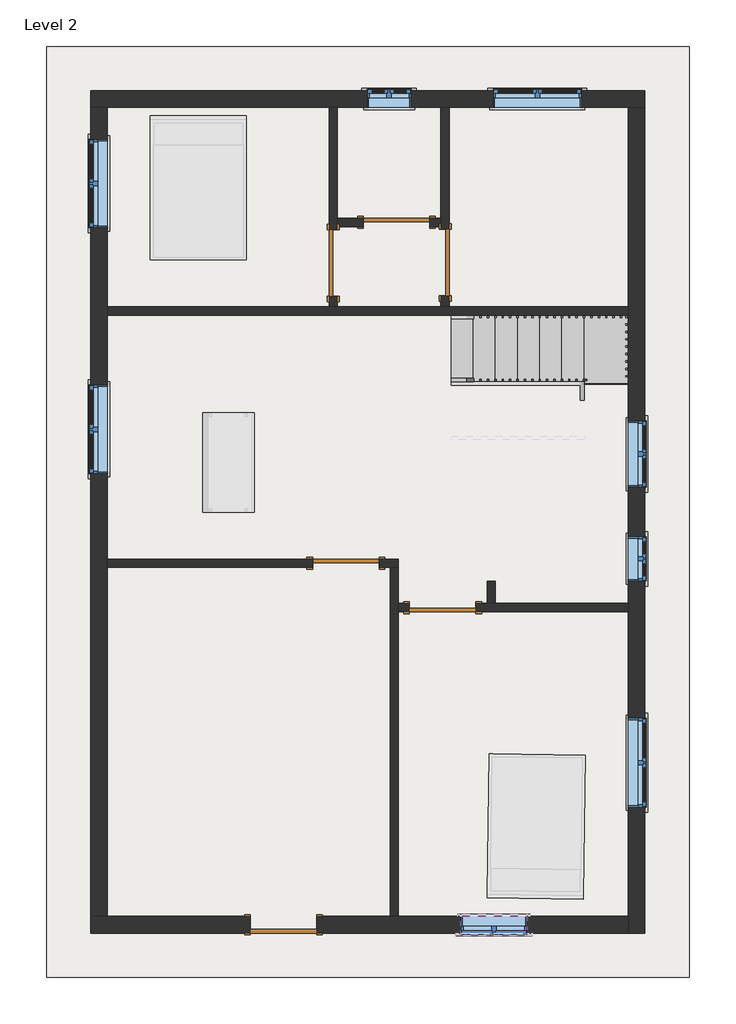
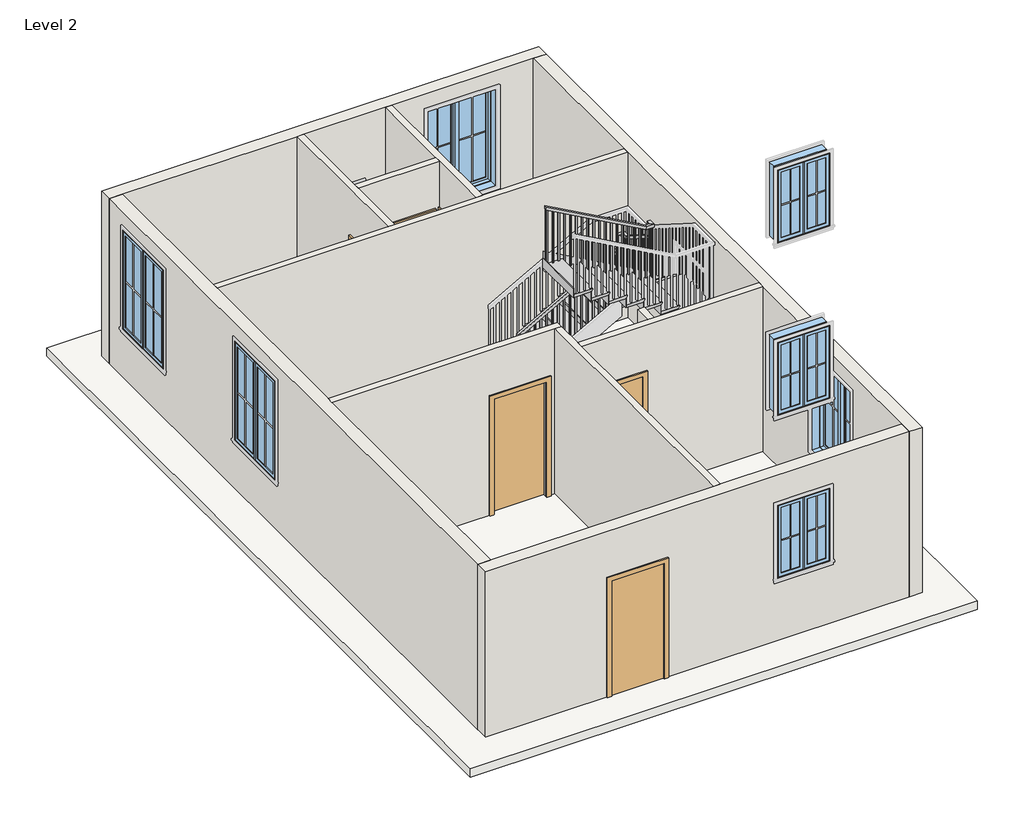
# One storey, part 1 of 2: 12 walls, 10 windows, 6 doors, 1 railing, 1 slab, 1 stair flight.
"""IFC4 building model written with IfcOpenShell, lengths in millimetres."""

from ifc_helpers import new_model, si_unit, frame, origin, place, context, project, spatial, polyline, outline, extrude, faceted_brep, transform, mapped, element, save
from components import door_e5f9f3c4, door_305aa2a5, door_0ca8825f, stair_flight_91d3489d, window_c417fced, window_79f73a1a, window_6ca1769e

model = new_model("IFC4")

# Units and contexts
model_context = context("Model", 3, world=origin())
ifc_project = project(units=[si_unit("LENGTHUNIT", "METRE", prefix="MILLI")], contexts=[model_context])

# Site, building, storey
site = spatial("IfcSite", under=ifc_project)
building = spatial("IfcBuilding", under=site)
storey = spatial("IfcBuildingStorey", under=building, Name="Level 2", Elevation=3048.0)

# Doors
placement = place(None, origin())
door_shape = door_e5f9f3c4(model_context)
element("IfcDoor", 1, ObjectType="Single-Flush : 36\" x 84\"", at=placement, inside=storey, context=model_context, shape_type="MappedRepresentation", body=[
    mapped(door_shape, transform((5727.7, 12245.5823212, 3048.0), x_axis=(1.0, 0.0, 0.0), y_axis=(0.0, 1.0, 0.0), z_axis=(0.0, 0.0, 1.0))),
])
element("IfcDoor", 2, ObjectType="Single-Flush : 36\" x 84\"", at=placement, inside=storey, context=model_context, shape_type="MappedRepresentation", body=[
    mapped(door_shape, transform((6394.45, 11693.1323212, 3048.0), x_axis=(0.0, -1.0, 0.0), y_axis=(1.0, 0.0, 0.0), z_axis=(0.0, 0.0, 1.0))),
])
element("IfcDoor", 3, ObjectType="Single-Flush : 36\" x 84\"", at=placement, inside=storey, context=model_context, shape_type="MappedRepresentation", body=[
    mapped(door_shape, transform((6362.7, 6949.6823212, 3048.0), x_axis=(-1.0, 0.0, 0.0), y_axis=(0.0, -1.0, 0.0), z_axis=(0.0, 0.0, 1.0))),
])
element("IfcDoor", 4, ObjectType="Single-Flush : 36\" x 84\"", at=placement, inside=storey, context=model_context, shape_type="MappedRepresentation", body=[
    mapped(door_shape, transform((5029.2, 7559.2823212, 3048.0), x_axis=(1.0, 0.0, 0.0), y_axis=(0.0, 1.0, 0.0), z_axis=(0.0, 0.0, 1.0))),
])
door_2_shape = door_305aa2a5(model_context)
element("IfcDoor", 5, ObjectType="Single-Flush : 36\" x 84\"", at=placement, inside=storey, context=model_context, shape_type="MappedRepresentation", body=[
    mapped(door_2_shape, transform((4857.75, 11689.9573212, 3048.0), x_axis=(0.0, -1.0, 0.0), y_axis=(1.0, 0.0, 0.0), z_axis=(0.0, 0.0, 1.0))),
])
door_3_shape = door_0ca8825f(model_context)
element("IfcDoor", 6, ObjectType="Single-Flush : 36\" x 84\"", at=placement, inside=storey, context=model_context, shape_type="MappedRepresentation", body=[
    mapped(door_3_shape, transform((4171.95, 2587.2323212, 3048.0), x_axis=(-1.0, 0.0, 0.0), y_axis=(0.0, -1.0, 0.0), z_axis=(0.0, 0.0, 1.0))),
])

# Railing
element("IfcRailing", 7, ObjectType="Handrail - Rectangular", at=placement, inside=storey, context=model_context, shape_type="SolidModel", body=[
    faceted_brep([(6477.0, 10105.6323212, 4131.7333333), (6477.0, 10105.6323212, 4073.620221), (6477.0, 10054.8323212, 4073.620221), (6477.0, 10054.8323212, 4131.7333333), (8229.6, 10105.6323212, 5105.4), (8280.4, 10105.6323212, 5075.5091099), (8280.4, 10054.8323212, 5075.5091099), (8229.6, 10054.8323212, 5105.4), (8229.6, 10105.6323212, 5365.447619), (8280.4, 10105.6323212, 5314.647619), (8280.4, 10054.8323212, 5314.647619), (8229.6, 10054.8323212, 5365.447619), (8356.6, 10105.6323212, 5365.447619), (8356.6, 10105.6323212, 5314.647619), (8305.8, 10054.8323212, 5314.647619), (8305.8, 10054.8323212, 5365.447619), (8356.6, 9978.6323212, 5365.447619), (8356.6, 9963.8676405, 5314.647619), (8305.8, 9963.8676405, 5314.647619), (8305.8, 9978.6323212, 5365.447619), (8356.6, 9330.9323212, 5776.6857143), (8356.6, 9280.1323212, 5748.7652821), (8305.8, 9280.1323212, 5748.7652821), (8305.8, 9330.9323212, 5776.6857143), (8356.6, 9330.9323212, 6036.7333333), (8356.6, 9280.1323212, 5985.9333333), (8305.8, 9280.1323212, 5985.9333333), (8305.8, 9330.9323212, 6036.7333333), (8356.6, 9203.9323212, 6036.7333333), (8356.6, 9203.9323212, 5985.9333333), (8305.8, 9254.7323212, 5985.9333333), (8305.8, 9254.7323212, 6036.7333333), (8229.6, 9203.9323212, 6036.7333333), (8216.4363978, 9203.9323212, 5985.9333333), (8216.4363978, 9254.7323212, 5985.9333333), (8229.6, 9254.7323212, 6036.7333333), (6477.0, 9203.9323212, 7010.4), (6477.0, 9254.7323212, 7010.4), (6477.0, 9254.7323212, 6952.2868876), (6477.0, 9203.9323212, 6952.2868876)], [[[0, 1, 2, 3]], [[1, 0, 4, 5]], [[2, 1, 5, 6]], [[3, 2, 6, 7]], [[0, 3, 7, 4]], [[5, 4, 8, 9]], [[6, 5, 9, 10]], [[7, 6, 10, 11]], [[4, 7, 11, 8]], [[9, 8, 12, 13]], [[10, 9, 13, 14]], [[11, 10, 14, 15]], [[8, 11, 15, 12]], [[13, 12, 16, 17]], [[14, 13, 17, 18]], [[15, 14, 18, 19]], [[12, 15, 19, 16]], [[17, 16, 20, 21]], [[18, 17, 21, 22]], [[19, 18, 22, 23]], [[16, 19, 23, 20]], [[21, 20, 24, 25]], [[22, 21, 25, 26]], [[23, 22, 26, 27]], [[20, 23, 27, 24]], [[25, 24, 28, 29]], [[26, 25, 29, 30]], [[27, 26, 30, 31]], [[24, 27, 31, 28]], [[29, 28, 32, 33]], [[30, 29, 33, 34]], [[31, 30, 34, 35]], [[28, 31, 35, 32]], [[36, 37, 38, 39]], [[33, 32, 36, 39]], [[34, 33, 39, 38]], [[35, 34, 38, 37]], [[32, 35, 37, 36]]]),
    extrude(outline(polyline([(6932.8841099, 6511.925), (6943.4674432, 6492.875), (5926.6666667, 6492.875), (5926.6666667, 6511.925), (6932.8841099, 6511.925)])), frame((0.0, 9219.8073212, 0.0), z_axis=(0.0, 1.0, 0.0), x_axis=(0.0, 0.0, 1.0)), (0.0, 0.0, 1.0), 19.05),
    extrude(outline(polyline([(6876.4396654, 6613.525), (6887.0229988, 6594.475), (5926.6666667, 6594.475), (5926.6666667, 6613.525), (6876.4396654, 6613.525)])), frame((0.0, 9219.8073212, 0.0), z_axis=(0.0, 1.0, 0.0), x_axis=(0.0, 0.0, 1.0)), (0.0, 0.0, 1.0), 19.05),
    extrude(outline(polyline([(6819.995221, 6715.125), (6830.5785543, 6696.075), (5926.6666667, 6696.075), (5926.6666667, 6715.125), (6819.995221, 6715.125)])), frame((0.0, 9219.8073212, 0.0), z_axis=(0.0, 1.0, 0.0), x_axis=(0.0, 0.0, 1.0)), (0.0, 0.0, 1.0), 19.05),
    extrude(outline(polyline([(6763.5507765, 6816.725), (6774.1341099, 6797.675), (5757.3333333, 6797.675), (5757.3333333, 6816.725), (6763.5507765, 6816.725)])), frame((0.0, 9219.8073212, 0.0), z_axis=(0.0, 1.0, 0.0), x_axis=(0.0, 0.0, 1.0)), (0.0, 0.0, 1.0), 19.05),
    extrude(outline(polyline([(6707.1063321, 6918.325), (6717.6896654, 6899.275), (5757.3333333, 6899.275), (5757.3333333, 6918.325), (6707.1063321, 6918.325)])), frame((0.0, 9219.8073212, 0.0), z_axis=(0.0, 1.0, 0.0), x_axis=(0.0, 0.0, 1.0)), (0.0, 0.0, 1.0), 19.05),
    extrude(outline(polyline([(6650.6618876, 7019.925), (6661.245221, 7000.875), (5757.3333333, 7000.875), (5757.3333333, 7019.925), (6650.6618876, 7019.925)])), frame((0.0, 9219.8073212, 0.0), z_axis=(0.0, 1.0, 0.0), x_axis=(0.0, 0.0, 1.0)), (0.0, 0.0, 1.0), 19.05),
    extrude(outline(polyline([(6594.2174432, 7121.525), (6604.8007765, 7102.475), (5588.0, 7102.475), (5588.0, 7121.525), (6594.2174432, 7121.525)])), frame((0.0, 9219.8073212, 0.0), z_axis=(0.0, 1.0, 0.0), x_axis=(0.0, 0.0, 1.0)), (0.0, 0.0, 1.0), 19.05),
    extrude(outline(polyline([(6537.7729988, 7223.125), (6548.3563321, 7204.075), (5588.0, 7204.075), (5588.0, 7223.125), (6537.7729988, 7223.125)])), frame((0.0, 9219.8073212, 0.0), z_axis=(0.0, 1.0, 0.0), x_axis=(0.0, 0.0, 1.0)), (0.0, 0.0, 1.0), 19.05),
    extrude(outline(polyline([(6481.3285543, 7324.725), (6491.9118876, 7305.675), (5588.0, 7305.675), (5588.0, 7324.725), (6481.3285543, 7324.725)])), frame((0.0, 9219.8073212, 0.0), z_axis=(0.0, 1.0, 0.0), x_axis=(0.0, 0.0, 1.0)), (0.0, 0.0, 1.0), 19.05),
    extrude(outline(polyline([(6424.8841099, 7426.325), (6435.4674432, 7407.275), (5418.6666667, 7407.275), (5418.6666667, 7426.325), (6424.8841099, 7426.325)])), frame((0.0, 9219.8073212, 0.0), z_axis=(0.0, 1.0, 0.0), x_axis=(0.0, 0.0, 1.0)), (0.0, 0.0, 1.0), 19.05),
    extrude(outline(polyline([(6368.4396654, 7527.925), (6379.0229988, 7508.875), (5418.6666667, 7508.875), (5418.6666667, 7527.925), (6368.4396654, 7527.925)])), frame((0.0, 9219.8073212, 0.0), z_axis=(0.0, 1.0, 0.0), x_axis=(0.0, 0.0, 1.0)), (0.0, 0.0, 1.0), 19.05),
    extrude(outline(polyline([(6311.995221, 7629.525), (6322.5785543, 7610.475), (5418.6666667, 7610.475), (5418.6666667, 7629.525), (6311.995221, 7629.525)])), frame((0.0, 9219.8073212, 0.0), z_axis=(0.0, 1.0, 0.0), x_axis=(0.0, 0.0, 1.0)), (0.0, 0.0, 1.0), 19.05),
    extrude(outline(polyline([(6255.5507765, 7731.125), (6266.1341099, 7712.075), (5249.3333333, 7712.075), (5249.3333333, 7731.125), (6255.5507765, 7731.125)])), frame((0.0, 9219.8073212, 0.0), z_axis=(0.0, 1.0, 0.0), x_axis=(0.0, 0.0, 1.0)), (0.0, 0.0, 1.0), 19.05),
    extrude(outline(polyline([(6199.1063321, 7832.725), (6209.6896654, 7813.675), (5249.3333333, 7813.675), (5249.3333333, 7832.725), (6199.1063321, 7832.725)])), frame((0.0, 9219.8073212, 0.0), z_axis=(0.0, 1.0, 0.0), x_axis=(0.0, 0.0, 1.0)), (0.0, 0.0, 1.0), 19.05),
    extrude(outline(polyline([(6142.6618876, 7934.325), (6153.245221, 7915.275), (5249.3333333, 7915.275), (5249.3333333, 7934.325), (6142.6618876, 7934.325)])), frame((0.0, 9219.8073212, 0.0), z_axis=(0.0, 1.0, 0.0), x_axis=(0.0, 0.0, 1.0)), (0.0, 0.0, 1.0), 19.05),
    extrude(outline(polyline([(6086.2174432, 8035.925), (6096.8007765, 8016.875), (5080.0, 8016.875), (5080.0, 8035.925), (6086.2174432, 8035.925)])), frame((0.0, 9219.8073212, 0.0), z_axis=(0.0, 1.0, 0.0), x_axis=(0.0, 0.0, 1.0)), (0.0, 0.0, 1.0), 19.05),
    extrude(outline(polyline([(6029.7729988, 8137.525), (6040.3563321, 8118.475), (5080.0, 8118.475), (5080.0, 8137.525), (6029.7729988, 8137.525)])), frame((0.0, 9219.8073212, 0.0), z_axis=(0.0, 1.0, 0.0), x_axis=(0.0, 0.0, 1.0)), (0.0, 0.0, 1.0), 19.05),
    extrude(outline(polyline([(5973.3285543, 8239.125), (5983.9118876, 8220.075), (5080.0, 8220.075), (5080.0, 8239.125), (5973.3285543, 8239.125)])), frame((0.0, 9219.8073212, 0.0), z_axis=(0.0, 1.0, 0.0), x_axis=(0.0, 0.0, 1.0)), (0.0, 0.0, 1.0), 19.05),
    extrude(outline(polyline([(8321.675, 9276.9573212), (8340.725, 9276.9573212), (8340.725, 9257.9073212), (8321.675, 9257.9073212), (8321.675, 9276.9573212)])), frame((0.0, 0.0, 4741.3333333), z_axis=(0.0, 0.0, 1.0), x_axis=(1.0, 0.0, 0.0)), (0.0, 0.0, 1.0), 1244.6),
    extrude(outline(polyline([(9359.5073212, 5698.3684567), (9378.5573212, 5686.2732186), (9378.5573212, 4741.3333333), (9359.5073212, 4741.3333333), (9359.5073212, 5698.3684567)])), frame((8321.675, 0.0, 0.0), z_axis=(1.0, 0.0, 0.0), x_axis=(0.0, 1.0, 0.0)), (0.0, 0.0, 1.0), 19.05),
    extrude(outline(polyline([(9461.1073212, 5633.8605202), (9480.1573212, 5621.7652821), (9480.1573212, 4741.3333333), (9461.1073212, 4741.3333333), (9461.1073212, 5633.8605202)])), frame((8321.675, 0.0, 0.0), z_axis=(1.0, 0.0, 0.0), x_axis=(0.0, 1.0, 0.0)), (0.0, 0.0, 1.0), 19.05),
    extrude(outline(polyline([(9562.7073212, 5569.3525837), (9581.7573212, 5557.2573456), (9581.7573212, 4572.0), (9562.7073212, 4572.0), (9562.7073212, 5569.3525837)])), frame((8321.675, 0.0, 0.0), z_axis=(1.0, 0.0, 0.0), x_axis=(0.0, 1.0, 0.0)), (0.0, 0.0, 1.0), 19.05),
    extrude(outline(polyline([(9664.3073212, 5504.8446472), (9683.3573212, 5492.7494091), (9683.3573212, 4572.0), (9664.3073212, 4572.0), (9664.3073212, 5504.8446472)])), frame((8321.675, 0.0, 0.0), z_axis=(1.0, 0.0, 0.0), x_axis=(0.0, 1.0, 0.0)), (0.0, 0.0, 1.0), 19.05),
    extrude(outline(polyline([(9765.9073212, 5440.3367107), (9784.9573212, 5428.2414726), (9784.9573212, 4402.6666667), (9765.9073212, 4402.6666667), (9765.9073212, 5440.3367107)])), frame((8321.675, 0.0, 0.0), z_axis=(1.0, 0.0, 0.0), x_axis=(0.0, 1.0, 0.0)), (0.0, 0.0, 1.0), 19.05),
    extrude(outline(polyline([(9867.5073212, 5375.8287742), (9886.5573212, 5363.7335361), (9886.5573212, 4402.6666667), (9867.5073212, 4402.6666667), (9867.5073212, 5375.8287742)])), frame((8321.675, 0.0, 0.0), z_axis=(1.0, 0.0, 0.0), x_axis=(0.0, 1.0, 0.0)), (0.0, 0.0, 1.0), 19.05),
    extrude(outline(polyline([(9969.1073212, 5311.3208377), (9988.1573212, 5299.2255996), (9988.1573212, 4402.6666667), (9969.1073212, 4402.6666667), (9969.1073212, 5311.3208377)])), frame((8321.675, 0.0, 0.0), z_axis=(1.0, 0.0, 0.0), x_axis=(0.0, 1.0, 0.0)), (0.0, 0.0, 1.0), 19.05),
    extrude(outline(polyline([(8296.275, 10070.7073212), (8296.275, 10089.7573212), (8315.325, 10089.7573212), (8315.325, 10070.7073212), (8296.275, 10070.7073212)])), frame((0.0, 0.0, 4233.3333333), z_axis=(0.0, 0.0, 1.0), x_axis=(1.0, 0.0, 0.0)), (0.0, 0.0, 1.0), 1081.3142857),
    extrude(outline(polyline([(5038.4674432, 8213.725), (5027.8841099, 8194.675), (4064.0, 8194.675), (4064.0, 8213.725), (5038.4674432, 8213.725)])), frame((0.0, 10070.7073212, 0.0), z_axis=(0.0, 1.0, 0.0), x_axis=(0.0, 0.0, 1.0)), (0.0, 0.0, 1.0), 19.05),
    extrude(outline(polyline([(4982.0229988, 8112.125), (4971.4396654, 8093.075), (4064.0, 8093.075), (4064.0, 8112.125), (4982.0229988, 8112.125)])), frame((0.0, 10070.7073212, 0.0), z_axis=(0.0, 1.0, 0.0), x_axis=(0.0, 0.0, 1.0)), (0.0, 0.0, 1.0), 19.05),
    extrude(outline(polyline([(4925.5785543, 8010.525), (4914.995221, 7991.475), (4064.0, 7991.475), (4064.0, 8010.525), (4925.5785543, 8010.525)])), frame((0.0, 10070.7073212, 0.0), z_axis=(0.0, 1.0, 0.0), x_axis=(0.0, 0.0, 1.0)), (0.0, 0.0, 1.0), 19.05),
    extrude(outline(polyline([(4869.1341099, 7908.925), (4858.5507765, 7889.875), (3894.6666667, 7889.875), (3894.6666667, 7908.925), (4869.1341099, 7908.925)])), frame((0.0, 10070.7073212, 0.0), z_axis=(0.0, 1.0, 0.0), x_axis=(0.0, 0.0, 1.0)), (0.0, 0.0, 1.0), 19.05),
    extrude(outline(polyline([(4812.6896654, 7807.325), (4802.1063321, 7788.275), (3894.6666667, 7788.275), (3894.6666667, 7807.325), (4812.6896654, 7807.325)])), frame((0.0, 10070.7073212, 0.0), z_axis=(0.0, 1.0, 0.0), x_axis=(0.0, 0.0, 1.0)), (0.0, 0.0, 1.0), 19.05),
    extrude(outline(polyline([(4756.245221, 7705.725), (4745.6618876, 7686.675), (3894.6666667, 7686.675), (3894.6666667, 7705.725), (4756.245221, 7705.725)])), frame((0.0, 10070.7073212, 0.0), z_axis=(0.0, 1.0, 0.0), x_axis=(0.0, 0.0, 1.0)), (0.0, 0.0, 1.0), 19.05),
    extrude(outline(polyline([(4699.8007765, 7604.125), (4689.2174432, 7585.075), (3725.3333333, 7585.075), (3725.3333333, 7604.125), (4699.8007765, 7604.125)])), frame((0.0, 10070.7073212, 0.0), z_axis=(0.0, 1.0, 0.0), x_axis=(0.0, 0.0, 1.0)), (0.0, 0.0, 1.0), 19.05),
    extrude(outline(polyline([(4643.3563321, 7502.525), (4632.7729988, 7483.475), (3725.3333333, 7483.475), (3725.3333333, 7502.525), (4643.3563321, 7502.525)])), frame((0.0, 10070.7073212, 0.0), z_axis=(0.0, 1.0, 0.0), x_axis=(0.0, 0.0, 1.0)), (0.0, 0.0, 1.0), 19.05),
    extrude(outline(polyline([(4586.9118876, 7400.925), (4576.3285543, 7381.875), (3725.3333333, 7381.875), (3725.3333333, 7400.925), (4586.9118876, 7400.925)])), frame((0.0, 10070.7073212, 0.0), z_axis=(0.0, 1.0, 0.0), x_axis=(0.0, 0.0, 1.0)), (0.0, 0.0, 1.0), 19.05),
    extrude(outline(polyline([(4530.4674432, 7299.325), (4519.8841099, 7280.275), (3556.0, 7280.275), (3556.0, 7299.325), (4530.4674432, 7299.325)])), frame((0.0, 10070.7073212, 0.0), z_axis=(0.0, 1.0, 0.0), x_axis=(0.0, 0.0, 1.0)), (0.0, 0.0, 1.0), 19.05),
    extrude(outline(polyline([(4474.0229988, 7197.725), (4463.4396654, 7178.675), (3556.0, 7178.675), (3556.0, 7197.725), (4474.0229988, 7197.725)])), frame((0.0, 10070.7073212, 0.0), z_axis=(0.0, 1.0, 0.0), x_axis=(0.0, 0.0, 1.0)), (0.0, 0.0, 1.0), 19.05),
    extrude(outline(polyline([(4417.5785543, 7096.125), (4406.995221, 7077.075), (3556.0, 7077.075), (3556.0, 7096.125), (4417.5785543, 7096.125)])), frame((0.0, 10070.7073212, 0.0), z_axis=(0.0, 1.0, 0.0), x_axis=(0.0, 0.0, 1.0)), (0.0, 0.0, 1.0), 19.05),
    extrude(outline(polyline([(4361.1341099, 6994.525), (4350.5507765, 6975.475), (3386.6666667, 6975.475), (3386.6666667, 6994.525), (4361.1341099, 6994.525)])), frame((0.0, 10070.7073212, 0.0), z_axis=(0.0, 1.0, 0.0), x_axis=(0.0, 0.0, 1.0)), (0.0, 0.0, 1.0), 19.05),
    extrude(outline(polyline([(4304.6896654, 6892.925), (4294.1063321, 6873.875), (3386.6666667, 6873.875), (3386.6666667, 6892.925), (4304.6896654, 6892.925)])), frame((0.0, 10070.7073212, 0.0), z_axis=(0.0, 1.0, 0.0), x_axis=(0.0, 0.0, 1.0)), (0.0, 0.0, 1.0), 19.05),
    extrude(outline(polyline([(4248.245221, 6791.325), (4237.6618876, 6772.275), (3386.6666667, 6772.275), (3386.6666667, 6791.325), (4248.245221, 6791.325)])), frame((0.0, 10070.7073212, 0.0), z_axis=(0.0, 1.0, 0.0), x_axis=(0.0, 0.0, 1.0)), (0.0, 0.0, 1.0), 19.05),
    extrude(outline(polyline([(4191.8007765, 6689.725), (4181.2174432, 6670.675), (3217.3333333, 6670.675), (3217.3333333, 6689.725), (4191.8007765, 6689.725)])), frame((0.0, 10070.7073212, 0.0), z_axis=(0.0, 1.0, 0.0), x_axis=(0.0, 0.0, 1.0)), (0.0, 0.0, 1.0), 19.05),
    extrude(outline(polyline([(4135.3563321, 6588.125), (4124.7729988, 6569.075), (3217.3333333, 6569.075), (3217.3333333, 6588.125), (4135.3563321, 6588.125)])), frame((0.0, 10070.7073212, 0.0), z_axis=(0.0, 1.0, 0.0), x_axis=(0.0, 0.0, 1.0)), (0.0, 0.0, 1.0), 19.05),
    extrude(outline(polyline([(8321.675, 9238.8573212), (8340.725, 9238.8573212), (8340.725, 9219.8073212), (8321.675, 9219.8073212), (8321.675, 9238.8573212)])), frame((0.0, 0.0, 4910.6666667), z_axis=(0.0, 0.0, 1.0), x_axis=(1.0, 0.0, 0.0)), (0.0, 0.0, 1.0), 1075.2666667),
    extrude(outline(polyline([(8321.675, 10070.7073212), (8321.675, 10089.7573212), (8340.725, 10089.7573212), (8340.725, 10070.7073212), (8321.675, 10070.7073212)])), frame((0.0, 0.0, 4233.3333333), z_axis=(0.0, 0.0, 1.0), x_axis=(1.0, 0.0, 0.0)), (0.0, 0.0, 1.0), 1081.3142857),
    extrude(outline(polyline([(6941.7035543, 6496.05), (6952.2868876, 6477.0), (5926.6666667, 6477.0), (5926.6666667, 6496.05), (6941.7035543, 6496.05)])), frame((0.0, 9219.8073212, 0.0), z_axis=(0.0, 1.0, 0.0), x_axis=(0.0, 0.0, 1.0)), (0.0, 0.0, 1.0), 19.05),
    extrude(outline(polyline([(4084.2035543, 6496.05), (4073.620221, 6477.0), (3217.3333333, 6477.0), (3217.3333333, 6496.05), (4084.2035543, 6496.05)])), frame((0.0, 10070.7073212, 0.0), z_axis=(0.0, 1.0, 0.0), x_axis=(0.0, 0.0, 1.0)), (0.0, 0.0, 1.0), 19.05),
])

# Slab
element("IfcSlab", 8, ObjectType="Generic - 12\"", at=placement, inside=storey, context=model_context, shape_type="SweptSolid", body=[
    extrude(outline(polyline([(9753.6, 14664.9323212), (9753.6, 1863.3323212), (914.4, 1863.3323212), (914.4, 14664.9323212), (9753.6, 14664.9323212)])), frame((0.0, 0.0, 2895.6), z_axis=(0.0, 0.0, 1.0), x_axis=(1.0, 0.0, 0.0)), (0.0, 0.0, 1.0), 152.4),
])

# Stair flight
stair_flight_shape = stair_flight_91d3489d(model_context)
element("IfcStairFlight", 9, ObjectType="2\" Tread 1\" Nosing 1/4\" Riser", at=placement, inside=storey, context=model_context, shape_type="MappedRepresentation", body=[
    mapped(stair_flight_shape, transform((0.0, 0.0, 0.0), x_axis=(1.0, 0.0, 0.0), y_axis=(0.0, 1.0, 0.0), z_axis=(0.0, 0.0, 1.0))),
])

# Walls
element("IfcWall", 10, ObjectType="Generic - 5\"", at=placement, inside=storey, context=model_context, shape_type="Brep", body=[
    faceted_brep([(4800.6, 11232.7573212, 5181.6), (4800.6, 11232.7573212, 3048.0), (4800.6, 11083.5323212, 3048.0), (4800.6, 11083.5323212, 6096.0), (4800.6, 13826.7323212, 6096.0), (4800.6, 13826.7323212, 3048.0), (4800.6, 12147.1573212, 3048.0), (4800.6, 12147.1573212, 5181.6), (4914.9, 11083.5323212, 3048.0), (4914.9, 11232.7573212, 3048.0), (4914.9, 11232.7573212, 5181.6), (4914.9, 12147.1573212, 5181.6), (4914.9, 12147.1573212, 3048.0), (4914.9, 12188.4323212, 3048.0), (4914.9, 12302.7323212, 3048.0), (4914.9, 13826.7323212, 3048.0), (4914.9, 13826.7323212, 6096.0), (4914.9, 12302.7323212, 6096.0), (4914.9, 12188.4323212, 6096.0), (4914.9, 11083.5323212, 6096.0)], [[[0, 1, 2, 3, 4, 5, 6, 7]], [[8, 9, 10, 11, 12, 13, 14, 15, 16, 17, 18, 19]], [[6, 5, 15, 14, 13, 12]], [[2, 1, 9, 8]], [[4, 3, 19, 18, 17, 16]], [[5, 4, 16, 15]], [[3, 2, 8, 19]], [[10, 9, 1, 0]], [[11, 10, 0, 7]], [[12, 11, 7, 6]]]),
])
element("IfcWall", 11, ObjectType="Generic - 5\"", at=placement, inside=storey, context=model_context, shape_type="Brep", body=[
    faceted_brep([(6337.3, 11235.9323212, 5181.6), (6337.3, 11235.9323212, 3048.0), (6337.3, 11083.5323212, 3048.0), (6337.3, 11083.5323212, 6096.0), (6337.3, 12188.4323212, 6096.0), (6337.3, 12302.7323212, 6096.0), (6337.3, 13826.7323212, 6096.0), (6337.3, 13826.7323212, 3048.0), (6337.3, 12302.7323212, 3048.0), (6337.3, 12188.4323212, 3048.0), (6337.3, 12150.3323212, 3048.0), (6337.3, 12150.3323212, 5181.6), (6451.6, 11083.5323212, 3048.0), (6451.6, 11235.9323212, 3048.0), (6451.6, 11235.9323212, 5181.6), (6451.6, 12150.3323212, 5181.6), (6451.6, 12150.3323212, 3048.0), (6451.6, 13826.7323212, 3048.0), (6451.6, 13826.7323212, 6096.0), (6451.6, 11083.5323212, 6096.0)], [[[0, 1, 2, 3, 4, 5, 6, 7, 8, 9, 10, 11]], [[12, 13, 14, 15, 16, 17, 18, 19]], [[2, 1, 13, 12]], [[10, 9, 8, 7, 17, 16]], [[6, 5, 4, 3, 19, 18]], [[7, 6, 18, 17]], [[3, 2, 12, 19]], [[14, 13, 1, 0]], [[15, 14, 0, 11]], [[16, 15, 11, 10]]]),
])
element("IfcWall", 12, ObjectType="Generic - 5\"", at=placement, inside=storey, context=model_context, shape_type="SweptSolid", body=[
    extrude(outline(polyline([(5181.6, 6184.9), (3048.0, 6184.9), (3048.0, 6337.3), (6096.0, 6337.3), (6096.0, 4914.9), (3048.0, 4914.9), (3048.0, 5270.5), (5181.6, 5270.5), (5181.6, 6184.9)])), frame((0.0, 12188.4323212, 0.0), z_axis=(0.0, 1.0, 0.0), x_axis=(0.0, 0.0, 1.0)), (0.0, 0.0, 1.0), 114.3),
])
element("IfcWall", 13, ObjectType="Generic - 5\"", at=placement, inside=storey, context=model_context, shape_type="Brep", body=[
    faceted_brep([(1752.6, 10969.2323212, 3048.0), (8915.4, 10969.2323212, 3048.0), (8915.4, 10969.2323212, 6096.0), (1752.6, 10969.2323212, 6096.0), (1752.6, 11083.5323212, 3048.0), (1752.6, 11083.5323212, 6096.0), (4800.6, 11083.5323212, 6096.0), (4914.9, 11083.5323212, 6096.0), (6337.3, 11083.5323212, 6096.0), (6451.6, 11083.5323212, 6096.0), (8915.4, 11083.5323212, 6096.0), (8915.4, 11083.5323212, 3048.0), (6451.6, 11083.5323212, 3048.0), (6337.3, 11083.5323212, 3048.0), (4914.9, 11083.5323212, 3048.0), (4800.6, 11083.5323212, 3048.0)], [[[0, 1, 2, 3]], [[4, 5, 6, 7, 8, 9, 10, 11, 12, 13, 14, 15]], [[1, 0, 4, 15, 14, 13, 12, 11]], [[3, 2, 10, 9, 8, 7, 6, 5]], [[2, 1, 11, 10]], [[0, 3, 5, 4]]]),
])
element("IfcWall", 14, ObjectType="Generic - 5\"", at=placement, inside=storey, context=model_context, shape_type="Brep", body=[
    faceted_brep([(5486.4, 7502.1323212, 5181.6), (5486.4, 7502.1323212, 3048.0), (5638.8, 7502.1323212, 3048.0), (5753.1, 7502.1323212, 3048.0), (5753.1, 7502.1323212, 6096.0), (5638.8, 7502.1323212, 6096.0), (1752.6, 7502.1323212, 6096.0), (1752.6, 7502.1323212, 3048.0), (4572.0, 7502.1323212, 3048.0), (4572.0, 7502.1323212, 5181.6), (5753.1, 7616.4323212, 3048.0), (5486.4, 7616.4323212, 3048.0), (5486.4, 7616.4323212, 5181.6), (4572.0, 7616.4323212, 5181.6), (4572.0, 7616.4323212, 3048.0), (1752.6, 7616.4323212, 3048.0), (1752.6, 7616.4323212, 6096.0), (5753.1, 7616.4323212, 6096.0)], [[[0, 1, 2, 3, 4, 5, 6, 7, 8, 9]], [[10, 11, 12, 13, 14, 15, 16, 17]], [[8, 7, 15, 14]], [[3, 2, 1, 11, 10]], [[6, 5, 4, 17, 16]], [[7, 6, 16, 15]], [[4, 3, 10, 17]], [[12, 11, 1, 0]], [[13, 12, 0, 9]], [[14, 13, 9, 8]]]),
])
element("IfcWall", 15, ObjectType="Generic - 5\"", at=placement, inside=storey, context=model_context, shape_type="Brep", body=[
    faceted_brep([(5638.8, 7502.1323212, 3048.0), (5638.8, 2701.5323212, 3048.0), (5638.8, 2701.5323212, 6096.0), (5638.8, 7502.1323212, 6096.0), (5753.1, 7502.1323212, 3048.0), (5753.1, 7502.1323212, 6096.0), (5753.1, 7006.8323212, 6096.0), (5753.1, 6892.5323212, 6096.0), (5753.1, 2701.5323212, 6096.0), (5753.1, 2701.5323212, 3048.0), (5753.1, 6892.5323212, 3048.0), (5753.1, 7006.8323212, 3048.0)], [[[0, 1, 2, 3]], [[4, 5, 6, 7, 8, 9, 10, 11]], [[1, 0, 4, 11, 10, 9]], [[3, 2, 8, 7, 6, 5]], [[0, 3, 5, 4]], [[2, 1, 9, 8]]]),
])
element("IfcWall", 16, ObjectType="Generic - 5\"", at=placement, inside=storey, context=model_context, shape_type="Brep", body=[
    faceted_brep([(5905.5, 7006.8323212, 5181.6), (5905.5, 7006.8323212, 3048.0), (5753.1, 7006.8323212, 3048.0), (5753.1, 7006.8323212, 6096.0), (6972.3, 7006.8323212, 6096.0), (7086.6, 7006.8323212, 6096.0), (8915.4, 7006.8323212, 6096.0), (8915.4, 7006.8323212, 3048.0), (7086.6, 7006.8323212, 3048.0), (6972.3, 7006.8323212, 3048.0), (6819.9, 7006.8323212, 3048.0), (6819.9, 7006.8323212, 5181.6), (5753.1, 6892.5323212, 3048.0), (5905.5, 6892.5323212, 3048.0), (5905.5, 6892.5323212, 5181.6), (6819.9, 6892.5323212, 5181.6), (6819.9, 6892.5323212, 3048.0), (8915.4, 6892.5323212, 3048.0), (8915.4, 6892.5323212, 6096.0), (5753.1, 6892.5323212, 6096.0)], [[[0, 1, 2, 3, 4, 5, 6, 7, 8, 9, 10, 11]], [[12, 13, 14, 15, 16, 17, 18, 19]], [[2, 1, 13, 12]], [[10, 9, 8, 7, 17, 16]], [[6, 5, 4, 3, 19, 18]], [[7, 6, 18, 17]], [[3, 2, 12, 19]], [[14, 13, 1, 0]], [[15, 14, 0, 11]], [[16, 15, 11, 10]]]),
])
element("IfcWall", 17, ObjectType="Generic - 5\"", at=placement, inside=storey, context=model_context, shape_type="SweptSolid", body=[
    extrude(outline(polyline([(7086.6, 7311.6323212), (7086.6, 7006.8323212), (6972.3, 7006.8323212), (6972.3, 7311.6323212), (7086.6, 7311.6323212)])), frame((0.0, 0.0, 3048.0), z_axis=(0.0, 0.0, 1.0), x_axis=(1.0, 0.0, 0.0)), (0.0, 0.0, 1.0), 3048.0),
])
element("IfcWall", 18, ObjectType="Generic - 8\"", at=placement, inside=storey, context=model_context, shape_type="Brep", body=[
    faceted_brep([(1524.0, 13826.7323212, 3048.0), (1752.6, 13826.7323212, 3048.0), (4800.6, 13826.7323212, 3048.0), (4914.9, 13826.7323212, 3048.0), (6337.3, 13826.7323212, 3048.0), (6451.6, 13826.7323212, 3048.0), (8915.4, 13826.7323212, 3048.0), (9144.0, 13826.7323212, 3048.0), (9144.0, 13826.7323212, 6096.0), (8915.4, 13826.7323212, 6096.0), (6451.6, 13826.7323212, 6096.0), (6337.3, 13826.7323212, 6096.0), (4914.9, 13826.7323212, 6096.0), (4800.6, 13826.7323212, 6096.0), (1752.6, 13826.7323212, 6096.0), (1524.0, 13826.7323212, 6096.0), (8274.05, 13826.7323212, 5791.2), (8274.05, 13826.7323212, 3962.4), (7054.85, 13826.7323212, 3962.4), (7054.85, 13826.7323212, 5791.2), (5930.9, 13826.7323212, 4876.8), (5930.9, 13826.7323212, 3962.4), (5321.3, 13826.7323212, 3962.4), (5321.3, 13826.7323212, 4876.8), (1524.0, 14055.3323212, 3048.0), (1524.0, 14055.3323212, 6096.0), (9144.0, 14055.3323212, 6096.0), (9144.0, 14055.3323212, 3048.0), (8274.05, 14055.3323212, 5791.2), (7054.85, 14055.3323212, 5791.2), (7054.85, 14055.3323212, 3962.4), (8274.05, 14055.3323212, 3962.4), (5930.9, 14055.3323212, 4876.8), (5321.3, 14055.3323212, 4876.8), (5321.3, 14055.3323212, 3962.4), (5930.9, 14055.3323212, 3962.4)], [[[0, 1, 2, 3, 4, 5, 6, 7, 8, 9, 10, 11, 12, 13, 14, 15], [16, 17, 18, 19], [20, 21, 22, 23]], [[24, 25, 26, 27], [28, 29, 30, 31], [32, 33, 34, 35]], [[7, 6, 5, 4, 3, 2, 1, 0, 24, 27]], [[15, 14, 13, 12, 11, 10, 9, 8, 26, 25]], [[8, 7, 27, 26]], [[0, 15, 25, 24]], [[17, 16, 28, 31]], [[18, 17, 31, 30]], [[19, 18, 30, 29]], [[16, 19, 29, 28]], [[21, 20, 32, 35]], [[22, 21, 35, 34]], [[23, 22, 34, 33]], [[20, 23, 33, 32]]]),
])
element("IfcWall", 19, ObjectType="Generic - 8\"", at=placement, inside=storey, context=model_context, shape_type="Brep", body=[
    faceted_brep([(8915.4, 13826.7323212, 3048.0), (8915.4, 11083.5323212, 3048.0), (8915.4, 10969.2323212, 3048.0), (8915.4, 7006.8323212, 3048.0), (8915.4, 6892.5323212, 3048.0), (8915.4, 2701.5323212, 3048.0), (8915.4, 2472.9323212, 3048.0), (8915.4, 2472.9323212, 6096.0), (8915.4, 2701.5323212, 6096.0), (8915.4, 6892.5323212, 6096.0), (8915.4, 7006.8323212, 6096.0), (8915.4, 10969.2323212, 6096.0), (8915.4, 11083.5323212, 6096.0), (8915.4, 13826.7323212, 6096.0), (8915.4, 4206.4823212, 5791.2), (8915.4, 4206.4823212, 3962.4), (8915.4, 5425.6823212, 3962.4), (8915.4, 5425.6823212, 5791.2), (8915.4, 7315.6010712, 4876.8), (8915.4, 7315.6010712, 3962.4), (8915.4, 7925.2010712, 3962.4), (8915.4, 7925.2010712, 4876.8), (8915.4, 8602.8899384, 5308.6), (8915.4, 8602.8899384, 3962.4), (8915.4, 9517.2899384, 3962.4), (8915.4, 9517.2899384, 5308.6), (9144.0, 13826.7323212, 3048.0), (9144.0, 13826.7323212, 6096.0), (9144.0, 2472.9323212, 6096.0), (9144.0, 2472.9323212, 3048.0), (9144.0, 4206.4823212, 5791.2), (9144.0, 5425.6823212, 5791.2), (9144.0, 5425.6823212, 3962.4), (9144.0, 4206.4823212, 3962.4), (9144.0, 7315.6010712, 4876.8), (9144.0, 7925.2010712, 4876.8), (9144.0, 7925.2010712, 3962.4), (9144.0, 7315.6010712, 3962.4), (9144.0, 8602.8899384, 5308.6), (9144.0, 9517.2899384, 5308.6), (9144.0, 9517.2899384, 3962.4), (9144.0, 8602.8899384, 3962.4)], [[[0, 1, 2, 3, 4, 5, 6, 7, 8, 9, 10, 11, 12, 13], [14, 15, 16, 17], [18, 19, 20, 21], [22, 23, 24, 25]], [[26, 27, 28, 29], [30, 31, 32, 33], [34, 35, 36, 37], [38, 39, 40, 41]], [[6, 5, 4, 3, 2, 1, 0, 26, 29]], [[13, 12, 11, 10, 9, 8, 7, 28, 27]], [[0, 13, 27, 26]], [[7, 6, 29, 28]], [[15, 14, 30, 33]], [[16, 15, 33, 32]], [[17, 16, 32, 31]], [[14, 17, 31, 30]], [[19, 18, 34, 37]], [[20, 19, 37, 36]], [[21, 20, 36, 35]], [[18, 21, 35, 34]], [[23, 22, 38, 41]], [[24, 23, 41, 40]], [[25, 24, 40, 39]], [[22, 25, 39, 38]]]),
])
element("IfcWall", 20, ObjectType="Generic - 8\"", at=placement, inside=storey, context=model_context, shape_type="Brep", body=[
    faceted_brep([(3714.75, 2701.5323212, 5181.6), (3714.75, 2701.5323212, 3048.0), (1752.6, 2701.5323212, 3048.0), (1524.0, 2701.5323212, 3048.0), (1524.0, 2701.5323212, 6096.0), (1752.6, 2701.5323212, 6096.0), (5638.8, 2701.5323212, 6096.0), (5753.1, 2701.5323212, 6096.0), (8915.4, 2701.5323212, 6096.0), (8915.4, 2701.5323212, 3048.0), (5753.1, 2701.5323212, 3048.0), (5638.8, 2701.5323212, 3048.0), (4629.15, 2701.5323212, 3048.0), (4629.15, 2701.5323212, 5181.6), (6610.35, 2701.5323212, 5555.780542), (6610.35, 2701.5323212, 4209.580542), (7524.75, 2701.5323212, 4209.580542), (7524.75, 2701.5323212, 5555.780542), (1524.0, 2472.9323212, 3048.0), (3714.75, 2472.9323212, 3048.0), (3714.75, 2472.9323212, 5181.6), (4629.15, 2472.9323212, 5181.6), (4629.15, 2472.9323212, 3048.0), (8915.4, 2472.9323212, 3048.0), (8915.4, 2472.9323212, 6096.0), (1524.0, 2472.9323212, 6096.0), (6610.35, 2472.9323212, 5555.780542), (7524.75, 2472.9323212, 5555.780542), (7524.75, 2472.9323212, 4209.580542), (6610.35, 2472.9323212, 4209.580542)], [[[0, 1, 2, 3, 4, 5, 6, 7, 8, 9, 10, 11, 12, 13], [14, 15, 16, 17]], [[18, 19, 20, 21, 22, 23, 24, 25], [26, 27, 28, 29]], [[3, 2, 1, 19, 18]], [[12, 11, 10, 9, 23, 22]], [[8, 7, 6, 5, 4, 25, 24]], [[9, 8, 24, 23]], [[4, 3, 18, 25]], [[20, 19, 1, 0]], [[21, 20, 0, 13]], [[22, 21, 13, 12]], [[15, 14, 26, 29]], [[16, 15, 29, 28]], [[17, 16, 28, 27]], [[14, 17, 27, 26]]]),
])
element("IfcWall", 21, ObjectType="Generic - 8\"", at=placement, inside=storey, context=model_context, shape_type="Brep", body=[
    faceted_brep([(1752.6, 2701.5323212, 3048.0), (1752.6, 7502.1323212, 3048.0), (1752.6, 7616.4323212, 3048.0), (1752.6, 10969.2323212, 3048.0), (1752.6, 11083.5323212, 3048.0), (1752.6, 13826.7323212, 3048.0), (1752.6, 13826.7323212, 6096.0), (1752.6, 11083.5323212, 6096.0), (1752.6, 10969.2323212, 6096.0), (1752.6, 7616.4323212, 6096.0), (1752.6, 7502.1323212, 6096.0), (1752.6, 2701.5323212, 6096.0), (1752.6, 13390.2194306, 5791.2), (1752.6, 13390.2194306, 3962.4), (1752.6, 12171.0194306, 3962.4), (1752.6, 12171.0194306, 5791.2), (1752.6, 10010.3823212, 5791.2), (1752.6, 10010.3823212, 3962.4), (1752.6, 8791.1823212, 3962.4), (1752.6, 8791.1823212, 5791.2), (1524.0, 2701.5323212, 3048.0), (1524.0, 2701.5323212, 6096.0), (1524.0, 13826.7323212, 6096.0), (1524.0, 13826.7323212, 3048.0), (1524.0, 13390.2194306, 5791.2), (1524.0, 12171.0194306, 5791.2), (1524.0, 12171.0194306, 3962.4), (1524.0, 13390.2194306, 3962.4), (1524.0, 10010.3823212, 5791.2), (1524.0, 8791.1823212, 5791.2), (1524.0, 8791.1823212, 3962.4), (1524.0, 10010.3823212, 3962.4)], [[[0, 1, 2, 3, 4, 5, 6, 7, 8, 9, 10, 11], [12, 13, 14, 15], [16, 17, 18, 19]], [[20, 21, 22, 23], [24, 25, 26, 27], [28, 29, 30, 31]], [[5, 4, 3, 2, 1, 0, 20, 23]], [[11, 10, 9, 8, 7, 6, 22, 21]], [[6, 5, 23, 22]], [[0, 11, 21, 20]], [[13, 12, 24, 27]], [[14, 13, 27, 26]], [[15, 14, 26, 25]], [[12, 15, 25, 24]], [[17, 16, 28, 31]], [[18, 17, 31, 30]], [[19, 18, 30, 29]], [[16, 19, 29, 28]]]),
])

# Windows
window_shape = window_c417fced(model_context)
element("IfcWindow", 22, ObjectType="Window-Casement-Double : 24\" x 36\"", at=placement, inside=storey, context=model_context, shape_type="MappedRepresentation", body=[
    mapped(window_shape, transform((9029.7, 7620.4010712, 3048.0), x_axis=(0.0, -1.0, 0.0), y_axis=(1.0, 0.0, 0.0), z_axis=(0.0, 0.0, 1.0))),
])
element("IfcWindow", 23, ObjectType="Window-Casement-Double : 24\" x 36\"", at=placement, inside=storey, context=model_context, shape_type="MappedRepresentation", body=[
    mapped(window_shape, transform((5626.1, 13941.0323212, 3048.0), x_axis=(1.0, 0.0, 0.0), y_axis=(0.0, 1.0, 0.0), z_axis=(0.0, 0.0, 1.0))),
])
window_2_shape = window_79f73a1a(model_context)
element("IfcWindow", 24, ObjectType="Window-Casement-Double : 36\" x 53\"", at=placement, inside=storey, context=model_context, shape_type="MappedRepresentation", body=[
    mapped(window_2_shape, transform((9029.7, 9060.0899384, 3048.0), x_axis=(0.0, -1.0, 0.0), y_axis=(1.0, 0.0, 0.0), z_axis=(0.0, 0.0, 1.0))),
])
element("IfcWindow", 25, ObjectType="Window-Casement-Double : 36\" x 53\"", at=placement, inside=storey, context=model_context, shape_type="MappedRepresentation", body=[
    mapped(window_2_shape, transform((7067.55, 2587.2323212, 3295.180542), x_axis=(-1.0, 0.0, 0.0), y_axis=(0.0, -1.0, 0.0), z_axis=(0.0, 0.0, 1.0))),
])
element("IfcWindow", 26, ObjectType="Window-Casement-Double : 36\" x 53\"", at=placement, inside=storey, context=model_context, shape_type="MappedRepresentation", body=[
    mapped(window_2_shape, transform((7067.55, 2587.2323212, 6297.0110953), x_axis=(-1.0, 0.0, 0.0), y_axis=(0.0, -1.0, 0.0), z_axis=(0.0, 0.0, 1.0))),
])
element("IfcWindow", 27, ObjectType="Window-Casement-Double : 36\" x 53\"", at=placement, inside=storey, context=model_context, shape_type="MappedRepresentation", body=[
    mapped(window_2_shape, transform((7067.55, 2587.2323212, 9477.7345423), x_axis=(-1.0, 0.0, 0.0), y_axis=(0.0, -1.0, 0.0), z_axis=(0.0, 0.0, 1.0))),
])
window_3_shape = window_6ca1769e(model_context)
element("IfcWindow", 28, ObjectType="Window-Casement-Double : 48\" x 72\"", at=placement, inside=storey, context=model_context, shape_type="MappedRepresentation", body=[
    mapped(window_3_shape, transform((1638.3, 12780.6194306, 3048.0), x_axis=(0.0, 1.0, 0.0), y_axis=(-1.0, 0.0, 0.0), z_axis=(0.0, 0.0, 1.0))),
])
element("IfcWindow", 29, ObjectType="Window-Casement-Double : 48\" x 72\"", at=placement, inside=storey, context=model_context, shape_type="MappedRepresentation", body=[
    mapped(window_3_shape, transform((7664.45, 13941.0323212, 3048.0), x_axis=(1.0, 0.0, 0.0), y_axis=(0.0, 1.0, 0.0), z_axis=(0.0, 0.0, 1.0))),
])
element("IfcWindow", 30, ObjectType="Window-Casement-Double : 48\" x 72\"", at=placement, inside=storey, context=model_context, shape_type="MappedRepresentation", body=[
    mapped(window_3_shape, transform((9029.7, 4816.0823212, 3048.0), x_axis=(0.0, -1.0, 0.0), y_axis=(1.0, 0.0, 0.0), z_axis=(0.0, 0.0, 1.0))),
])
element("IfcWindow", 31, ObjectType="Window-Casement-Double : 48\" x 72\"", at=placement, inside=storey, context=model_context, shape_type="MappedRepresentation", body=[
    mapped(window_3_shape, transform((1638.3, 9400.7823212, 3048.0), x_axis=(0.0, 1.0, 0.0), y_axis=(-1.0, 0.0, 0.0), z_axis=(0.0, 0.0, 1.0))),
])

save(model, "model.ifc")

# Revit data of these elements
# Type "Single-Flush : 36\" x 84\""
#   Type Mark = "1"
#   Construction Type Id = "MDOOR"
#   Assembly Code = "C1020"
#   Analytic Construction = "Metal"
#   Thickness = 0' - 2"
#   Heat Transfer Coefficient (U) = 0.651978 BTU/(h·ft²·°F)
#   Height = 7' - 0"
#   Trim Projection Ext = 0' - 1"
#   Trim Projection Int = 0' - 1"
#   Trim Width = 0' - 3"
#   Width = 3' - 0"
#   Define Thermal Properties by = 1
#   Define Thermal Properties by = 1
#   Door Material = Door - Panel
#   Frame Material = Door - Frame
#   Visual Light Transmittance = 0
#   Solar Heat Gain Coefficient = 0
#   Function = (empty or 0)
#   Wall Closure = (empty or 0)
# Type "Handrail - Rectangular"
#   Assembly Code = "C2010400"
#   built-in parameter 1008612 = 0.0416667 (stored number, unit not read)
#   built-in parameter 1008611 = 0.0416667 (stored number, unit not read)
#   built-in parameter 1008609 = 0.333333 (stored number, unit not read)
#   built-in parameter 1008604 = 0.166667 (stored number, unit not read)
#   built-in parameter 1008603 = 0.166667 (stored number, unit not read)
#   Railing Height = 3' - 0"
#   built-in parameter 1008630 = 2
#   built-in parameter 1008610 = 2
#   built-in parameter 1008618 = Baluster - Square : 3/4"
# Type "Generic - 12\""
#   Assembly Code = "B1010"
#   Function = 0
#   Layers, outside or top first: 0' - 6" no material (function 1)
# Type "Generic - 5\""
#   Assembly Code = "B2010"
#   Layers, outside or top first: 0' - 4 1/2" no material (function 1)
# Type "Generic - 8\""
#   Assembly Code = "B2010"
#   Layers, outside or top first: 0' - 9" no material (function 1)
# Type "Window-Casement-Double : 24\" x 36\""
#   Type Mark = "14"
#   Fire Rating = "0.5h"
#   Assembly Code = "B2020100"
#   Analytic Construction = "Double glazing - domestic"
#   Frame Extension [instance default] = 0' - 0 1/4"
#   Window Inset [instance default] = 0' - 0"
#   Wall Thickness [instance default] = 0' - 6"
#   Interior Wall Closure [instance default] = 0' - 2 1/4"
#   Half Width = 1' - 0"
#   Visual Light Transmittance = 0.81
#   Thermal Resistance (R) = 1.8146 (h·ft²·°F)/BTU
#   Solar Heat Gain Coefficient = 0.76
#   Rough Width = 2' - 0 1/2"
#   Rough Height = 3' - 0 1/2"
#   Height = 3' - 0"
#   Heat Transfer Coefficient (U) = 0.5511 BTU/(h·ft²·°F)
#   Exterior Wall Closure [instance default] = 0' - 1 1/4"
#   Extension Jamb [instance default] = 0' - 2 1/4"
#   Default Sill Height = 3' - 0"
#   Width = 2' - 0"
#   Define Thermal Properties by = 0
#   Muntin Visibility = yes
#   Interior Trim Visibility [instance default] = yes
#   Exterior Trim Visibility [instance default] = yes
#   Extension Jamb Visibility [instance default] = yes
#   Interior Trim Material = Wood - Stained
#   Muntin Pattern = Muntin Pattern_2x2 : Muntin Pattern_2x2
#   Interior Trim = Trim-Window-Interior-Flat : Picture Frame
#   Interior Frame Material = Wood - Stained
#   Glass Panel Material = Glass
#   Exterior Trim Material = Clad - White
#   Exterior Trim = Trim-Window-Exterior-Flat : with Sill
#   Exterior Frame Material = Clad - White
#   Wall Closure = (empty or 0)
# Type "Window-Casement-Double : 36\" x 53\""
#   Type Mark = "15"
#   Fire Rating = "0.5h"
#   Assembly Code = "B2020100"
#   Analytic Construction = "Double glazing - domestic"
#   Frame Extension [instance default] = 0' - 0 1/4"
#   Window Inset [instance default] = 0' - 0"
#   Wall Thickness [instance default] = 0' - 6"
#   Interior Wall Closure [instance default] = 0' - 2 1/4"
#   Half Width = 1' - 6"
#   Visual Light Transmittance = 0.81
#   Thermal Resistance (R) = 1.8146 (h·ft²·°F)/BTU
#   Solar Heat Gain Coefficient = 0.76
#   Rough Width = 3' - 0 1/2"
#   Rough Height = 4' - 5 1/2"
#   Height = 4' - 5"
#   Heat Transfer Coefficient (U) = 0.5511 BTU/(h·ft²·°F)
#   Exterior Wall Closure [instance default] = 0' - 1 1/4"
#   Extension Jamb [instance default] = 0' - 2 1/4"
#   Default Sill Height = 3' - 0"
#   Width = 3' - 0"
#   Define Thermal Properties by = 0
#   Muntin Visibility = yes
#   Interior Trim Visibility [instance default] = yes
#   Exterior Trim Visibility [instance default] = yes
#   Extension Jamb Visibility [instance default] = yes
#   Interior Trim Material = Wood - Stained
#   Muntin Pattern = Muntin Pattern_2x2 : Muntin Pattern_2x2
#   Interior Trim = Trim-Window-Interior-Flat : Picture Frame
#   Interior Frame Material = Wood - Stained
#   Glass Panel Material = Glass
#   Exterior Trim Material = Clad - White
#   Exterior Trim = Trim-Window-Exterior-Flat : with Sill
#   Exterior Frame Material = Clad - White
#   Wall Closure = (empty or 0)
# Type "Window-Casement-Double : 48\" x 72\""
#   Type Mark = "17"
#   Fire Rating = "0.5h"
#   Assembly Code = "B2020100"
#   Analytic Construction = "Double glazing - domestic"
#   Frame Extension [instance default] = 0' - 0 1/4"
#   Window Inset [instance default] = 0' - 0"
#   Wall Thickness [instance default] = 0' - 6"
#   Interior Wall Closure [instance default] = 0' - 2 1/4"
#   Half Width = 2' - 0"
#   Visual Light Transmittance = 0.81
#   Thermal Resistance (R) = 1.8146 (h·ft²·°F)/BTU
#   Solar Heat Gain Coefficient = 0.76
#   Rough Width = 4' - 0 1/2"
#   Rough Height = 6' - 0 1/2"
#   Height = 6' - 0"
#   Heat Transfer Coefficient (U) = 0.5511 BTU/(h·ft²·°F)
#   Exterior Wall Closure [instance default] = 0' - 1 1/4"
#   Extension Jamb [instance default] = 0' - 2 1/4"
#   Default Sill Height = 3' - 0"
#   Width = 4' - 0"
#   Define Thermal Properties by = 0
#   Muntin Visibility = yes
#   Interior Trim Visibility [instance default] = yes
#   Exterior Trim Visibility [instance default] = yes
#   Extension Jamb Visibility [instance default] = yes
#   Interior Trim Material = Wood - Stained
#   Muntin Pattern = Muntin Pattern_2x2 : Muntin Pattern_2x2
#   Interior Trim = Trim-Window-Interior-Flat : Picture Frame
#   Interior Frame Material = Wood - Stained
#   Glass Panel Material = Glass
#   Exterior Trim Material = Clad - White
#   Exterior Trim = Trim-Window-Exterior-Flat : with Sill
#   Exterior Frame Material = Clad - White
#   Wall Closure = (empty or 0)
# Elements 1, 2, 3, 4, 5, 6 (IfcDoor, "Single-Flush : 36\" x 84\"")
#   Phase Created = New Construction
#   Materials on its faces: "Door - Frame", "Door - Panel"
# Element 7 (IfcRailing, "Handrail - Rectangular")
#   Phase Created = New Construction
# Element 8 (IfcSlab, "Generic - 12\"")
#   Height Offset From Level = 0' - 0"
#   Phase Created = New Construction
#   Materials on its faces: "Carpet (1)", "Default Floor"
# Element 9 (IfcStairFlight, "2\" Tread 1\" Nosing 1/4\" Riser")
#   Phase Created = New Construction
# Elements 10, 11, 12, 13, 14, 15, 16, 17 (IfcWall, "Generic - 5\"")
#   Top Offset = 0' - 0"
#   Base Offset = 0' - 0"
#   wall height = 10' - 0"
#   Phase Created = New Construction
#   Base Constraint = Level 2
#   Top Constraint = Level 3
#   Materials on its faces: "Default Wall"
# Elements 18, 19, 20, 21 (IfcWall, "Generic - 8\"")
#   Top Offset = 0' - 0"
#   Base Offset = 0' - 0"
#   Unconnected Height = 10' - 0"
#   wall height = 10' - 0"
#   Phase Created = New Construction
#   Base Constraint = Level 2
#   Materials on its faces: "Default Wall", "Wood - Stained"
# Element 22 (IfcWindow, "Window-Casement-Double : 24\" x 36\"")
#   Mark = "12"
#   Window Inset = 0' - 0"
#   Interior Wall Closure = 0' - 2 1/4"
#   Frame Extension = 0' - 0 1/4"
#   Exterior Wall Closure = 0' - 1 1/4"
#   Interior Trim Visibility = yes
#   Exterior Trim Visibility = yes
#   Phase Created = New Construction
#   Materials on its faces: "Wood - Stained", "Glass", "Clad - White"
# Element 23 (IfcWindow, "Window-Casement-Double : 24\" x 36\"")
#   Mark = "13"
#   Window Inset = 0' - 0"
#   Interior Wall Closure = 0' - 2 1/4"
#   Frame Extension = 0' - 0 1/4"
#   Exterior Wall Closure = 0' - 1 1/4"
#   Interior Trim Visibility = yes
#   Exterior Trim Visibility = yes
#   Phase Created = New Construction
#   Materials on its faces: "Wood - Stained", "Glass", "Clad - White"
# Element 24 (IfcWindow, "Window-Casement-Double : 36\" x 53\"")
#   Mark = "14"
#   Window Inset = 0' - 0"
#   Interior Wall Closure = 0' - 2 1/4"
#   Frame Extension = 0' - 0 1/4"
#   Exterior Wall Closure = 0' - 1 1/4"
#   Interior Trim Visibility = yes
#   Exterior Trim Visibility = yes
#   Phase Created = New Construction
#   Materials on its faces: "Wood - Stained", "Glass", "Clad - White"
# Element 25 (IfcWindow, "Window-Casement-Double : 36\" x 53\"")
#   Mark = "29"
#   Window Inset = 0' - 0"
#   Interior Wall Closure = 0' - 2 1/4"
#   Frame Extension = 0' - 0 1/4"
#   Exterior Wall Closure = 0' - 1 1/4"
#   Interior Trim Visibility = yes
#   Exterior Trim Visibility = yes
#   Phase Created = New Construction
#   Materials on its faces: "Wood - Stained", "Glass", "Clad - White"
# Element 26 (IfcWindow, "Window-Casement-Double : 36\" x 53\"")
#   Mark = "30"
#   Window Inset = 0' - 0"
#   Interior Wall Closure = 0' - 2 1/4"
#   Frame Extension = 0' - 0 1/4"
#   Exterior Wall Closure = 0' - 1 1/4"
#   Interior Trim Visibility = yes
#   Exterior Trim Visibility = yes
#   Phase Created = New Construction
#   Materials on its faces: "Wood - Stained", "Glass", "Clad - White"
# Element 27 (IfcWindow, "Window-Casement-Double : 36\" x 53\"")
#   Mark = "31"
#   Window Inset = 0' - 0"
#   Interior Wall Closure = 0' - 2 1/4"
#   Frame Extension = 0' - 0 1/4"
#   Exterior Wall Closure = 0' - 1 1/4"
#   Interior Trim Visibility = yes
#   Exterior Trim Visibility = yes
#   Phase Created = New Construction
#   Materials on its faces: "Wood - Stained", "Glass", "Clad - White"
# Element 28 (IfcWindow, "Window-Casement-Double : 48\" x 72\"")
#   Mark = "8"
#   Window Inset = 0' - 0"
#   Interior Wall Closure = 0' - 2 1/4"
#   Frame Extension = 0' - 0 1/4"
#   Exterior Wall Closure = 0' - 1 1/4"
#   Interior Trim Visibility = yes
#   Exterior Trim Visibility = yes
#   Phase Created = New Construction
#   Materials on its faces: "Wood - Stained", "Glass", "Clad - White"
# Element 29 (IfcWindow, "Window-Casement-Double : 48\" x 72\"")
#   Mark = "9"
#   Window Inset = 0' - 0"
#   Interior Wall Closure = 0' - 2 1/4"
#   Frame Extension = 0' - 0 1/4"
#   Exterior Wall Closure = 0' - 1 1/4"
#   Interior Trim Visibility = yes
#   Exterior Trim Visibility = yes
#   Phase Created = New Construction
#   Materials on its faces: "Wood - Stained", "Glass", "Clad - White"
# Element 30 (IfcWindow, "Window-Casement-Double : 48\" x 72\"")
#   Mark = "10"
#   Window Inset = 0' - 0"
#   Interior Wall Closure = 0' - 2 1/4"
#   Frame Extension = 0' - 0 1/4"
#   Exterior Wall Closure = 0' - 1 1/4"
#   Interior Trim Visibility = yes
#   Exterior Trim Visibility = yes
#   Phase Created = New Construction
#   Materials on its faces: "Wood - Stained", "Glass", "Clad - White"
# Element 31 (IfcWindow, "Window-Casement-Double : 48\" x 72\"")
#   Mark = "11"
#   Window Inset = 0' - 0"
#   Interior Wall Closure = 0' - 2 1/4"
#   Frame Extension = 0' - 0 1/4"
#   Exterior Wall Closure = 0' - 1 1/4"
#   Interior Trim Visibility = yes
#   Exterior Trim Visibility = yes
#   Phase Created = New Construction
#   Materials on its faces: "Wood - Stained", "Glass", "Clad - White"
# Materials
#   "Door - Panel": class "Wood", colour RGB 210 159 95, transparency 0, Cost = 0
#   "Door - Frame": colour RGB 118 70 51, transparency 0, Cost = 0
#   "Wood - Stained": class "Wood", colour RGB 224 178 126, transparency 0, Cost = 0
#   "Glass": class "Glass", colour RGB 0 128 192, transparency 0.75, Description = "Soda Lime Glass", Cost = 0
#   "Clad - White": class "Wood", colour RGB 242 242 238, transparency 0, Cost = 0
#   "Carpet (1)": class "Carpet", colour RGB 124 80 67, transparency 0, Description = "Interior finish", Cost = 0
#   "Default Floor": colour RGB 128 128 128, transparency 0, Cost = 0
#   "Default Wall": colour RGB 128 128 128, transparency 0, Cost = 0
